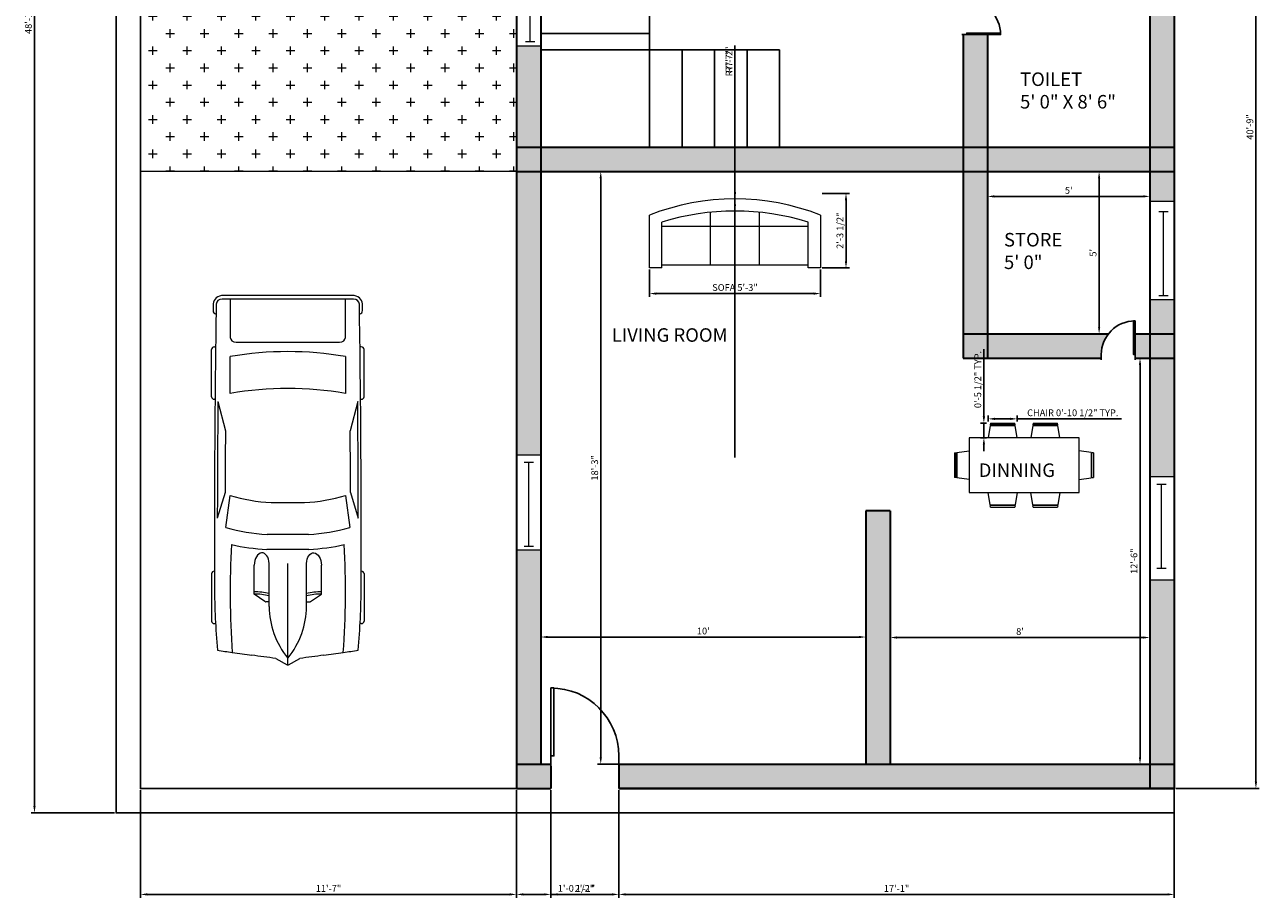
# Model space of a CAD drawing. Units: millimetres. Extents: x 2602 to 3574, y 848 to 1501.
# Tile 1 of 3: x 2602 to 3058, y 848 to 1172. Entities that reach past the tile are written whole.
import ezdxf

# ---------------------------------------------------------------- set-up
doc = ezdxf.new("R2010")
doc.units = ezdxf.units.MM
for name, color, linetype, lineweight in [('A-ANNO-DIMS', 170, 'Continuous', 18), ('A-AREA-IDEN', 200, 'Continuous', 18), ('A-WALL-PATT', 140, 'Continuous', 13), ('C-PROP', 140, 'Continuous', 25), ('C-SITE-VEHI', 90, 'Continuous', 13), ('doors', 10, 'Continuous', 25), ('furniture', 90, 'Continuous', 18), ('L-PLNT', 140, 'Continuous', 18), ('L-PLNT-PATT', 152, 'Continuous', 13), ('STAIRCASE', 30, 'Continuous', 25), ('walls', 140, 'Continuous', 35), ('windows', 40, 'Continuous', 18)]:
    doc.layers.add(name, color=color, linetype=linetype, lineweight=lineweight)
doc.styles.get("Standard").update_dxf_attribs({"font": 'arial.ttf'})
doc.dimstyles.new('ISO-25', dxfattribs={"dimtxt": 2.5, "dimasz": 2.5, "dimexe": 1.25, "dimexo": 0.625, "dimtad": 1, "dimdec": 0, "dimlunit": 3, "dimtxsty": 'Standard', "dimcen": 2.5, "dimadec": 0, "dimazin": 0, "dimtfac": 1, "dimtdec": 0, "dimtmove": 0, "dimatfit": 3, "dimfxl": 1, "dimarcsym": 0})

# ---------------------------------------------------------------- blocks, each defined once
blk = doc.blocks.new('*U2')
for p, q in [((0, 0), (0, -6)), ((40, 0), (40, -6))]:
    blk.add_line(p, q)
blk.add_lwpolyline([(0, 0), (0, 40), (1.75, 40), (1.75, 0)], close=True)
blk.add_arc((0, 0), 40, 0, 90)
blk = doc.blocks.new('*U4')
for p, q in [((0, 4), (0, 0)), ((0, 2), (36, 2)), ((36, 4), (36, 0))]:
    blk.add_line(p, q)
blk = doc.blocks.new('Sofa - Roundback 7 ft.')
for p, q in [((-36.000027, -34), (-36.000027, -11.4696)), ((-12.00002, -32.4421), (-12.00003, -6.5971)), ((11.99997, -32.4421), (11.99998, -6.5971)), ((35.99998, -34), (35.99998, -11.4696)), ((-35.999844, -13.3819), (35.9998, -13.3819)), ((-36.000027, -32.4421), (35.99998, -32.4421))]:
    blk.add_line(p, q)
for points in [[(-36.000027, -34), (-42.000027, -34), (-42.000027, -8)], [(41.99998, -8), (41.99998, -34), (35.99998, -34)]]:
    blk.add_lwpolyline(points)
for centre, radius, start, end in [((0, -114.25), 114.25, 68.43141, 111.5686), ((-0.00001, -127.1968), 121.1968, 72.72033, 107.2797)]:
    blk.add_arc(centre, radius, start, end)
blk = doc.blocks.new('*D13')
at = {"layer": 'A-ANNO-DIMS', "color": 0, "lineweight": -2, "transparency": 16777216}
for p, q in [((2993.44, 1117.36), (3000.35, 1117.36)), ((2999.1, 1114.86), (2999.1, 1059.86)), ((2993.44, 1057.36), (3000.35, 1057.36))]:
    blk.add_line(p, q, dxfattribs=at)
at = {"layer": 'A-ANNO-DIMS', "color": 0, "transparency": 16777216}
for points in [[(2998.69, 1114.86), (2999.52, 1114.86), (2999.1, 1117.36)], [(2998.69, 1059.86), (2999.52, 1059.86), (2999.1, 1057.36)]]:
    blk.add_solid(points, dxfattribs=at)
at = {"layer": 'Defpoints', "color": 0, "transparency": 16777216}
for p in [(2992.82, 1117.36), (2992.82, 1057.36), (2999.1, 1057.36)]:
    blk.add_point(p, dxfattribs=at)
at = {"layer": 'A-ANNO-DIMS', "color": 0, "transparency": 16777216, "insert": (2997.21, 1087.36), "char_height": 2.5, "attachment_point": 5, "rotation": 90}
blk.add_mtext("5'", dxfattribs=at)
blk = doc.blocks.new('*D14')
at = {"layer": 'A-ANNO-DIMS', "color": 0, "lineweight": -2, "transparency": 16777216}
for p, q in [((2957.88, 1110.38), (2957.88, 1106.94)), ((3017.88, 1110.38), (3017.88, 1106.94)), ((3015.38, 1108.19), (2960.38, 1108.19))]:
    blk.add_line(p, q, dxfattribs=at)
at = {"layer": 'A-ANNO-DIMS', "color": 0, "transparency": 16777216}
for points in [[(2960.38, 1108.61), (2960.38, 1107.77), (2957.88, 1108.19)], [(3015.38, 1108.61), (3015.38, 1107.77), (3017.88, 1108.19)]]:
    blk.add_solid(points, dxfattribs=at)
at = {"layer": 'Defpoints', "color": 0, "transparency": 16777216}
for p in [(2957.88, 1111.01), (3017.88, 1111.01), (2957.88, 1108.19)]:
    blk.add_point(p, dxfattribs=at)
at = {"layer": 'A-ANNO-DIMS', "color": 0, "transparency": 16777216, "insert": (2987.88, 1110.09), "char_height": 2.5, "attachment_point": 5}
blk.add_mtext("5'", dxfattribs=at)
blk = doc.blocks.new('*D15')
at = {"layer": 'A-ANNO-DIMS', "color": 0, "lineweight": -2, "transparency": 16777216}
for p, q in [((2921.88, 937.69), (2921.88, 946.41)), ((3015.38, 945.16), (2924.38, 945.16)), ((3017.88, 937.69), (3017.88, 946.41))]:
    blk.add_line(p, q, dxfattribs=at)
at = {"layer": 'A-ANNO-DIMS', "color": 0, "transparency": 16777216}
for points in [[(2924.38, 945.57), (2924.38, 944.74), (2921.88, 945.16)], [(3015.38, 945.57), (3015.38, 944.74), (3017.88, 945.16)]]:
    blk.add_solid(points, dxfattribs=at)
at = {"layer": 'Defpoints', "color": 0, "transparency": 16777216}
for p in [(2921.88, 945.16), (2921.88, 937.07), (3017.88, 937.07)]:
    blk.add_point(p, dxfattribs=at)
at = {"layer": 'A-ANNO-DIMS', "color": 0, "transparency": 16777216, "insert": (2969.88, 947.06), "char_height": 2.5, "attachment_point": 5}
blk.add_mtext("8'", dxfattribs=at)
blk = doc.blocks.new('*D16')
at = {"layer": 'A-ANNO-DIMS', "color": 0, "lineweight": -2, "transparency": 16777216}
for p, q in [((3014.62, 1048.36), (3012.96, 1048.36)), ((3014.21, 1045.86), (3014.21, 900.86)), ((3014.62, 898.36), (3012.96, 898.36))]:
    blk.add_line(p, q, dxfattribs=at)
at = {"layer": 'A-ANNO-DIMS', "color": 0, "transparency": 16777216}
for points in [[(3013.8, 1045.86), (3014.63, 1045.86), (3014.21, 1048.36)], [(3013.8, 900.86), (3014.63, 900.86), (3014.21, 898.36)]]:
    blk.add_solid(points, dxfattribs=at)
at = {"layer": 'Defpoints', "color": 0, "transparency": 16777216}
for p in [(3015.24, 1048.36), (3014.21, 898.36), (3015.24, 898.36)]:
    blk.add_point(p, dxfattribs=at)
at = {"layer": 'A-ANNO-DIMS', "color": 0, "transparency": 16777216, "insert": (3012.31, 973.36), "char_height": 2.5, "attachment_point": 5, "rotation": 90}
blk.add_mtext('12\'-6"', dxfattribs=at)
blk = doc.blocks.new('*D17')
at = {"layer": 'A-ANNO-DIMS', "color": 0, "lineweight": -2, "transparency": 16777216}
for p, q in [((2792.88, 975.8), (2792.88, 944.09)), ((2912.88, 975.8), (2912.88, 944.09)), ((2910.38, 945.34), (2795.38, 945.34))]:
    blk.add_line(p, q, dxfattribs=at)
at = {"layer": 'A-ANNO-DIMS', "color": 0, "transparency": 16777216}
for points in [[(2795.38, 945.76), (2795.38, 944.92), (2792.88, 945.34)], [(2910.38, 945.76), (2910.38, 944.92), (2912.88, 945.34)]]:
    blk.add_solid(points, dxfattribs=at)
at = {"layer": 'Defpoints', "color": 0, "transparency": 16777216}
for p in [(2792.88, 976.43), (2912.88, 976.43), (2792.88, 945.34)]:
    blk.add_point(p, dxfattribs=at)
at = {"layer": 'A-ANNO-DIMS', "color": 0, "transparency": 16777216, "insert": (2852.88, 947.24), "char_height": 2.5, "attachment_point": 5}
blk.add_mtext("10'", dxfattribs=at)
blk = doc.blocks.new('*D18')
at = {"layer": 'A-ANNO-DIMS', "color": 0, "lineweight": -2, "transparency": 16777216}
for p, q in [((2830.28, 1117.36), (2813.75, 1117.36)), ((2815, 900.86), (2815, 1114.86)), ((2830.28, 898.36), (2813.75, 898.36))]:
    blk.add_line(p, q, dxfattribs=at)
at = {"layer": 'A-ANNO-DIMS', "color": 0, "transparency": 16777216}
for points in [[(2814.58, 1114.86), (2815.41, 1114.86), (2815, 1117.36)], [(2814.58, 900.86), (2815.41, 900.86), (2815, 898.36)]]:
    blk.add_solid(points, dxfattribs=at)
at = {"layer": 'Defpoints', "color": 0, "transparency": 16777216}
for p in [(2815, 1117.36), (2830.91, 1117.36), (2830.91, 898.36)]:
    blk.add_point(p, dxfattribs=at)
at = {"layer": 'A-ANNO-DIMS', "color": 0, "transparency": 16777216, "insert": (2813.09, 1007.86), "char_height": 2.5, "attachment_point": 5, "rotation": 90}
blk.add_mtext('18\'-3"', dxfattribs=at)
blk = doc.blocks.new('*U22')
for p, q in [((46.55, 38.89), (22.35, 38.89)), ((136.7, 38.89), (160.9, 38.89)), ((21.1, 37.41), (21.1, 36.83)), ((47.8, 37.39), (47.8, 37.41)), ((70.03, 31.54), (86.41, 29.35)), ((87.99, 31.87), (74.76, 35.92)), ((134.31, 35.6), (119.29, 31.78)), ((135.45, 37.07), (135.45, 37.41)), ((162.15, 37.41), (162.15, 36.77)), ((186.47, -33.5), (186.47, 33.5)), ((188.4, -32.76), (188.4, 32.76)), ((138.42, 29.35), (157.25, 29.35)), ((164.52, 26.39), (164.52, -26.39)), ((186.47, 29.35), (167.01, 29.35)), ((32.27, 11.63), (36.13, 17.17)), ((36.13, 17.17), (50.94, 17.17)), ((29.77, 9.51), (51.68, 9.51)), ((32.12, 9.51), (32.12, 11.15)), ((58.92, -10.77), (58.92, 10.77)), ((66.55, -10.53), (66.55, 10.53)), ((82.74, 8.5), (82.74, -8.5)), ((186.47, -10.53), (186.47, 10.53)), ((3.27, 6.13), (0.1, 0.41)), ((0, 0), (51.68, 0)), ((0.1, -0.41), (3.27, -6.13)), ((29.77, -9.51), (51.68, -9.51)), ((32.12, -9.51), (32.12, -11.15)), ((32.27, -11.63), (36.13, -17.17)), ((36.13, -17.17), (50.94, -17.17)), ((86.41, -29.35), (70.03, -31.54)), ((157.25, -29.35), (138.42, -29.35)), ((167.01, -29.35), (186.47, -29.35)), ((21.1, -37.41), (21.1, -36.83)), ((47.8, -37.39), (47.8, -37.41)), ((87.99, -31.87), (74.76, -35.92)), ((134.31, -35.6), (119.29, -31.78)), ((135.45, -37.07), (135.45, -37.41)), ((162.15, -37.41), (162.15, -36.77)), ((46.55, -38.89), (22.35, -38.89)), ((136.7, -38.89), (160.9, -38.89))]:
    blk.add_line(p, q)
for centre, major_axis, ratio, start_param, end_param in [((22.35, 37.41), (0, -1.48), 0.842304, 3.141593, 4.712389), ((46.55, 37.41), (0, 1.48), 0.842304, -1.570796, 0), ((136.7, 37.41), (0, -1.48), 0.842304, 3.141593, 4.712389), ((160.9, 37.41), (0, 1.48), 0.842304, -1.570796, 0), ((180.63, 35.84), (0, 2.22), 0.842304, -0.013017, 1.249894), ((64.48, -10556.36), (0, 10595.31), 0.842304, -0.013397, -0.013017), ((183.98, 32.76), (0, -5.25), 0.842304, 1.570796, 3.128196), ((266.03, -27.52), (0, 313.31), 0.842304, 1.367076, 1.39176), ((41.19, -490.86), (0, 528.23), 0.842304, 0.00281, 0.075598), ((64.48, -10555.62), (0, 10593.03), 0.842304, -0.013397, 0.002797), ((135.29, 5.39), (0, 81.77), 0.842304, 1.245306, 1.50788), ((64.48, -10555.62), (0, -10591.55), 0.842304, 3.133765, 3.140441), ((95.79, -3666.35), (0, -3698.24), 0.842304, 3.134049, 3.144098), ((183.98, 33.5), (0, -2.96), 0.842304, 1.570796, 3.128196), ((259.18, -27.52), (0, -305.3), 0.842304, 4.528606, 4.561838), ((37.47, -593.96), (0, -623.33), 0.842304, 3.096046, 3.200911), ((134.4, 5.39), (0, -89.78), 0.842304, 4.449482, 4.652344), ((149.6, 2.8), (0, -79.58), 0.842304, 4.372215, 4.640744), ((17.08, 0), (0, 147.02), 0.842304, 4.511394, 4.913384), ((35.91, 0), (0, 147.02), 0.842304, 4.511394, 4.913384), ((167.01, 26.39), (0, 2.96), 0.842304, 0, 1.570796), ((-204.49, 52.4), (0, -250.96), 0.842304, 1.385369, 1.434372), ((13.04, 17.01), (0, 27.42), 0.842304, 4.435146, 4.718221), ((14.2, 17.01), (0, 27.42), 0.842304, 4.435146, 4.718221), ((50.79, 13.34), (6.34, -0.36), 0.603834, -1.395552, 1.581315), ((29.77, -46.66), (0, 56.17), 0.842304, 0, 0.590319), ((32.75, 11.15), (0, 0.74), 0.842304, 0.879714, 1.570796), ((0.62, 0), (0, -0.74), 0.842304, 4.131459, 5.293319), ((-204.49, -52.4), (0, 250.96), 0.842304, -1.434372, -1.385369), ((29.77, 46.66), (0, 56.17), 0.842304, 2.551274, 3.141593), ((32.75, -11.15), (0, -0.74), 0.842304, 4.712389, 5.403472), ((13.04, -17.01), (0, -27.42), 0.842304, 1.564964, 1.848039), ((14.2, -17.01), (0, -27.42), 0.842304, 1.564964, 1.848039), ((134.4, -5.39), (0, -89.78), 0.842304, -1.510751, -1.307889), ((135.29, -5.39), (0, -81.77), 0.842304, -1.50788, -1.245306), ((149.6, -2.8), (0, -79.58), 0.842304, -1.499151, -1.230623), ((259.18, 27.52), (0, 305.3), 0.842304, 1.721348, 1.754579), ((266.03, 27.52), (0, 313.31), 0.842304, 1.749832, 1.774517), ((37.47, 593.96), (0, -623.33), 0.842304, -0.059319, 0.045547), ((167.01, -26.39), (0, -2.96), 0.842304, 4.712389, 6.283185), ((41.19, 490.86), (0, -528.23), 0.842304, -0.075598, -0.00281), ((22.35, -37.41), (0, 1.48), 0.842304, 1.570796, 3.141593), ((64.48, 10555.62), (0, 10593.03), 0.842304, 3.138796, 3.15499), ((46.55, -37.41), (0, -1.48), 0.842304, 0, 1.570796), ((64.48, 10555.62), (0, -10591.55), 0.842304, 0.001152, 0.007828), ((95.79, 3666.35), (0, -3698.24), 0.842304, -0.002505, 0.007544), ((136.7, -37.41), (0, -1.48), 0.842304, -1.570796, 0), ((160.9, -37.41), (0, 1.48), 0.842304, 3.141593, 4.712389), ((180.63, -35.84), (0, -2.22), 0.842304, -1.249894, 0.013017), ((183.98, -33.5), (0, 2.96), 0.842304, 3.15499, 4.712389), ((183.98, -32.76), (0, -5.25), 0.842304, 0.013397, 1.570796), ((64.48, 10556.36), (0, 10595.31), 0.842304, 3.15461, 3.15499)]:
    blk.add_ellipse(centre, major_axis=major_axis, ratio=ratio, start_param=start_param, end_param=end_param)
at = {"extrusion": (0, 0, -1)}
blk.add_ellipse((50.79, -13.34), major_axis=(6.34, 0.36), ratio=0.603834, start_param=-1.395552, end_param=1.581315, dxfattribs=at)
blk = doc.blocks.new('CHAIR-DINING')
for p, q in [((0.84, 5.36), (0.75, 4.79)), ((9.95, 4.79), (0.75, 4.79)), ((0.84, 5.36), (9.86, 5.36)), ((9.95, 4.79), (9.86, 5.36)), ((0.71, 4.51), (0, 0)), ((0.71, 4.51), (9.99, 4.51)), ((10.7, 0), (9.99, 4.51))]:
    blk.add_line(p, q)
blk = doc.blocks.new('*D26')
at = {"layer": 'A-ANNO-DIMS', "color": 0, "lineweight": -2, "transparency": 16777216}
for p, q in [((2958.13, 1024.99), (2958.13, 1027.22)), ((2968.83, 1024.99), (2968.83, 1027.22)), ((2960.63, 1025.97), (2966.33, 1025.97)), ((2968.83, 1025.97), (3007.39, 1025.97))]:
    blk.add_line(p, q, dxfattribs=at)
at = {"layer": 'A-ANNO-DIMS', "color": 0, "transparency": 16777216}
for points in [[(2960.63, 1026.39), (2960.63, 1025.56), (2958.13, 1025.97)], [(2966.33, 1026.39), (2966.33, 1025.56), (2968.83, 1025.97)]]:
    blk.add_solid(points, dxfattribs=at)
at = {"layer": 'Defpoints', "color": 0, "transparency": 16777216}
for p in [(2958.13, 1024.37), (2968.83, 1025.97), (2968.83, 1024.37)]:
    blk.add_point(p, dxfattribs=at)
at = {"layer": 'A-ANNO-DIMS', "color": 0, "transparency": 16777216, "insert": (2989.36, 1027.89), "char_height": 2.5, "attachment_point": 5}
blk.add_mtext('CHAIR 0\'-10 1/2" TYP.', dxfattribs=at)
blk = doc.blocks.new('*D27')
at = {"layer": 'A-ANNO-DIMS', "color": 0, "lineweight": -2, "transparency": 16777216}
for p, q in [((2956.53, 1026.87), (2956.53, 1051.68)), ((2957.51, 1024.37), (2955.28, 1024.37)), ((2956.53, 1019.01), (2956.53, 1024.37)), ((2957.51, 1019.01), (2955.28, 1019.01)), ((2956.53, 1016.51), (2956.53, 1014.01))]:
    blk.add_line(p, q, dxfattribs=at)
at = {"layer": 'A-ANNO-DIMS', "color": 0, "transparency": 16777216}
for points in [[(2956.11, 1026.87), (2956.95, 1026.87), (2956.53, 1024.37)], [(2956.11, 1016.51), (2956.95, 1016.51), (2956.53, 1019.01)]]:
    blk.add_solid(points, dxfattribs=at)
at = {"layer": 'Defpoints', "color": 0, "transparency": 16777216}
for p in [(2956.53, 1024.37), (2958.13, 1024.37), (2958.13, 1019.01)]:
    blk.add_point(p, dxfattribs=at)
at = {"layer": 'A-ANNO-DIMS', "color": 0, "transparency": 16777216, "insert": (2954.61, 1040.52), "char_height": 2.5, "attachment_point": 5, "rotation": 90}
blk.add_mtext('0\'-5 1/2" TYP.', dxfattribs=at)
blk = doc.blocks.new('*D36')
at = {"layer": 'A-ANNO-DIMS', "color": 0, "lineweight": -2, "transparency": 16777216}
for p, q in [((2833.05, 1081.12), (2833.05, 1071.03)), ((2896.14, 1081.12), (2896.14, 1071.03)), ((2835.55, 1072.28), (2893.64, 1072.28))]:
    blk.add_line(p, q, dxfattribs=at)
at = {"layer": 'A-ANNO-DIMS', "color": 0, "transparency": 16777216}
for points in [[(2835.55, 1072.7), (2835.55, 1071.86), (2833.05, 1072.28)], [(2893.64, 1072.7), (2893.64, 1071.86), (2896.14, 1072.28)]]:
    blk.add_solid(points, dxfattribs=at)
at = {"layer": 'Defpoints', "color": 0, "transparency": 16777216}
for p in [(2833.05, 1081.74), (2896.14, 1081.74), (2896.14, 1072.28)]:
    blk.add_point(p, dxfattribs=at)
at = {"layer": 'A-ANNO-DIMS', "color": 0, "transparency": 16777216, "insert": (2864.59, 1074.2), "char_height": 2.5, "attachment_point": 5}
blk.add_mtext('SOFA 5\'-3"', dxfattribs=at)
blk = doc.blocks.new('*D37')
at = {"layer": 'A-ANNO-DIMS', "color": 0, "lineweight": -2, "transparency": 16777216}
for p, q in [((2896.76, 1109.28), (2906.85, 1109.28)), ((2905.6, 1084.24), (2905.6, 1106.78)), ((2896.76, 1081.74), (2906.85, 1081.74))]:
    blk.add_line(p, q, dxfattribs=at)
at = {"layer": 'A-ANNO-DIMS', "color": 0, "transparency": 16777216}
for points in [[(2905.18, 1106.78), (2906.01, 1106.78), (2905.6, 1109.28)], [(2905.18, 1084.24), (2906.01, 1084.24), (2905.6, 1081.74)]]:
    blk.add_solid(points, dxfattribs=at)
at = {"layer": 'Defpoints', "color": 0, "transparency": 16777216}
for p in [(2896.14, 1109.28), (2905.6, 1109.28), (2896.14, 1081.74)]:
    blk.add_point(p, dxfattribs=at)
at = {"layer": 'A-ANNO-DIMS', "color": 0, "transparency": 16777216, "insert": (2903.68, 1095.51), "char_height": 2.5, "attachment_point": 5, "rotation": 90}
blk.add_mtext('2\'-3 1/2"', dxfattribs=at)
blk = doc.blocks.new('*D41')
at = {"layer": 'A-ANNO-DIMS', "color": 0, "lineweight": -2, "transparency": 16777216}
for p, q in [((2635.33, 1467.39), (2604.55, 1467.39)), ((2605.8, 882.86), (2605.8, 1464.89)), ((2635.33, 880.36), (2604.55, 880.36))]:
    blk.add_line(p, q, dxfattribs=at)
at = {"layer": 'A-ANNO-DIMS', "color": 0, "transparency": 16777216}
for points in [[(2605.39, 1464.89), (2606.22, 1464.89), (2605.8, 1467.39)], [(2605.39, 882.86), (2606.22, 882.86), (2605.8, 880.36)]]:
    blk.add_solid(points, dxfattribs=at)
at = {"layer": 'Defpoints', "color": 0, "transparency": 16777216}
for p in [(2605.8, 1467.39), (2635.95, 1467.39), (2635.95, 880.36)]:
    blk.add_point(p, dxfattribs=at)
at = {"layer": 'A-ANNO-DIMS', "color": 0, "transparency": 16777216, "insert": (2603.9, 1173.88), "char_height": 2.5, "attachment_point": 5, "rotation": 90}
blk.add_mtext('48\'-11"', dxfattribs=at)
blk = doc.blocks.new('*D42')
at = {"layer": 'A-ANNO-DIMS', "color": 0, "lineweight": -2, "transparency": 16777216}
for p, q in [((3027.5, 1378.36), (3058.28, 1378.36)), ((3057.03, 891.86), (3057.03, 1375.86)), ((3027.5, 889.36), (3058.28, 889.36))]:
    blk.add_line(p, q, dxfattribs=at)
at = {"layer": 'A-ANNO-DIMS', "color": 0, "transparency": 16777216}
for points in [[(3056.61, 1375.86), (3057.44, 1375.86), (3057.03, 1378.36)], [(3056.61, 891.86), (3057.44, 891.86), (3057.03, 889.36)]]:
    blk.add_solid(points, dxfattribs=at)
at = {"layer": 'Defpoints', "color": 0, "transparency": 16777216}
for p in [(3026.88, 1378.36), (3057.03, 1378.36), (3026.88, 889.36)]:
    blk.add_point(p, dxfattribs=at)
at = {"layer": 'A-ANNO-DIMS', "color": 0, "transparency": 16777216, "insert": (3055.12, 1133.86), "char_height": 2.5, "attachment_point": 5, "rotation": 90}
blk.add_mtext('40\'-9"', dxfattribs=at)
blk = doc.blocks.new('*D44')
at = {"layer": 'A-ANNO-DIMS', "color": 0, "lineweight": -2, "transparency": 16777216}
for p, q in [((2644.95, 888.74), (2644.95, 848.96)), ((2783.88, 888.74), (2783.88, 848.96)), ((2647.45, 850.21), (2781.38, 850.21))]:
    blk.add_line(p, q, dxfattribs=at)
at = {"layer": 'A-ANNO-DIMS', "color": 0, "transparency": 16777216}
for points in [[(2647.45, 850.63), (2647.45, 849.8), (2644.95, 850.21)], [(2781.38, 850.63), (2781.38, 849.8), (2783.88, 850.21)]]:
    blk.add_solid(points, dxfattribs=at)
at = {"layer": 'Defpoints', "color": 0, "transparency": 16777216}
for p in [(2644.95, 889.36), (2783.88, 889.36), (2783.88, 850.21)]:
    blk.add_point(p, dxfattribs=at)
at = {"layer": 'A-ANNO-DIMS', "color": 0, "transparency": 16777216, "insert": (2714.42, 852.09), "char_height": 2.5, "attachment_point": 5}
blk.add_mtext('11\'-7"', dxfattribs=at)
blk = doc.blocks.new('*D45')
at = {"layer": 'A-ANNO-DIMS', "color": 0, "lineweight": -2, "transparency": 16777216}
for p, q in [((2783.88, 888.74), (2783.88, 848.96)), ((2796.6, 888.74), (2796.6, 848.96)), ((2786.38, 850.21), (2794.1, 850.21)), ((2796.6, 850.21), (2812.58, 850.21))]:
    blk.add_line(p, q, dxfattribs=at)
at = {"layer": 'A-ANNO-DIMS', "color": 0, "transparency": 16777216}
for points in [[(2786.38, 850.63), (2786.38, 849.8), (2783.88, 850.21)], [(2794.1, 850.63), (2794.1, 849.8), (2796.6, 850.21)]]:
    blk.add_solid(points, dxfattribs=at)
at = {"layer": 'Defpoints', "color": 0, "transparency": 16777216}
for p in [(2783.88, 889.36), (2796.6, 889.36), (2796.6, 850.21)]:
    blk.add_point(p, dxfattribs=at)
at = {"layer": 'A-ANNO-DIMS', "color": 0, "transparency": 16777216, "insert": (2805.84, 852.13), "char_height": 2.5, "attachment_point": 5}
blk.add_mtext('1\'-0 1/2"', dxfattribs=at)
blk = doc.blocks.new('*D46')
at = {"layer": 'A-ANNO-DIMS', "color": 0, "lineweight": -2, "transparency": 16777216}
for p, q in [((2796.6, 888.74), (2796.6, 848.96)), ((2821.68, 888.74), (2821.68, 848.96)), ((2799.1, 850.21), (2819.18, 850.21))]:
    blk.add_line(p, q, dxfattribs=at)
at = {"layer": 'A-ANNO-DIMS', "color": 0, "transparency": 16777216}
for points in [[(2799.1, 850.63), (2799.1, 849.8), (2796.6, 850.21)], [(2819.18, 850.63), (2819.18, 849.8), (2821.68, 850.21)]]:
    blk.add_solid(points, dxfattribs=at)
at = {"layer": 'Defpoints', "color": 0, "transparency": 16777216}
for p in [(2796.6, 889.36), (2821.68, 889.36), (2821.68, 850.21)]:
    blk.add_point(p, dxfattribs=at)
at = {"layer": 'A-ANNO-DIMS', "color": 0, "transparency": 16777216, "insert": (2809.14, 852.09), "char_height": 2.5, "attachment_point": 5}
blk.add_mtext('2\'-1"', dxfattribs=at)
blk = doc.blocks.new('*D47')
at = {"layer": 'A-ANNO-DIMS', "color": 0, "lineweight": -2, "transparency": 16777216}
for p, q in [((2821.68, 888.74), (2821.68, 848.96)), ((3026.88, 888.74), (3026.88, 848.96)), ((2824.18, 850.21), (3024.38, 850.21))]:
    blk.add_line(p, q, dxfattribs=at)
at = {"layer": 'A-ANNO-DIMS', "color": 0, "transparency": 16777216}
for points in [[(2824.18, 850.63), (2824.18, 849.8), (2821.68, 850.21)], [(3024.38, 850.63), (3024.38, 849.8), (3026.88, 850.21)]]:
    blk.add_solid(points, dxfattribs=at)
at = {"layer": 'Defpoints', "color": 0, "transparency": 16777216}
for p in [(2821.68, 889.36), (3026.88, 889.36), (3026.88, 850.21)]:
    blk.add_point(p, dxfattribs=at)
at = {"layer": 'A-ANNO-DIMS', "color": 0, "transparency": 16777216, "insert": (2924.28, 852.09), "char_height": 2.5, "attachment_point": 5}
blk.add_mtext('17\'-1"', dxfattribs=at)
blk = doc.blocks.new('*D57')
at = {"layer": 'A-ANNO-DIMS', "color": 0, "lineweight": -2, "transparency": 16777216}
for p, q in [((2864.59, 1162.53), (2864.59, 1105.27)), ((2864.59, 1011.75), (2864.59, 1102.77))]:
    blk.add_line(p, q, dxfattribs=at)
at = {"layer": 'A-ANNO-DIMS', "color": 0, "transparency": 16777216}
blk.add_solid([(2864.18, 1105.27), (2865.01, 1105.27), (2864.59, 1102.77)], dxfattribs=at)
at = {"layer": 'Defpoints', "color": 0, "transparency": 16777216}
for p in [(2864.59, 1102.77), (2864.59, 1011.75)]:
    blk.add_point(p, dxfattribs=at)
at = {"layer": 'A-ANNO-DIMS', "color": 0, "transparency": 16777216, "insert": (2862.72, 1157.39), "char_height": 2.5, "attachment_point": 5, "rotation": 89.9998}
blk.add_mtext('R7\'-7"', dxfattribs=at)
blk = doc.blocks.new('*D58')
at = {"layer": 'A-ANNO-DIMS', "color": 0, "lineweight": -2, "transparency": 16777216}
for p, q in [((2864.59, 1163.91), (2864.59, 1109.78)), ((2864.59, 1021.47), (2864.59, 1107.28))]:
    blk.add_line(p, q, dxfattribs=at)
at = {"layer": 'A-ANNO-DIMS', "color": 0, "transparency": 16777216}
blk.add_solid([(2864.18, 1109.78), (2865.01, 1109.78), (2864.59, 1107.28)], dxfattribs=at)
at = {"layer": 'Defpoints', "color": 0, "transparency": 16777216}
for p in [(2864.59, 1107.28), (2864.59, 1021.47)]:
    blk.add_point(p, dxfattribs=at)
at = {"layer": 'A-ANNO-DIMS', "color": 0, "transparency": 16777216, "insert": (2862.71, 1158.76), "char_height": 2.5, "attachment_point": 5, "rotation": 89.9998}
blk.add_mtext('R7\'-2"', dxfattribs=at)

msp = doc.modelspace()

# ---------------------------------------------------------------- hatches: boundary and pattern name
at = {"layer": 'A-WALL-PATT'}
h = msp.add_hatch(color=256, dxfattribs=at)
h.dxf.hatch_style = 1
h.paths.add_polyline_path([(2792.88, 1117.36), (2783.88, 1117.36), (2783.88, 1012.52), (2792.88, 1012.52)])
h.paths.add_polyline_path([(2957.88, 1117.36), (2948.88, 1117.36), (2948.88, 1057.36), (2957.88, 1057.36)])
h.paths.add_polyline_path([(2957.88, 1057.36), (2948.88, 1057.36), (2948.88, 1048.36), (2957.88, 1048.36)])
h.paths.add_polyline_path([(3002.51, 1057.36), (2957.88, 1057.36), (2957.88, 1048.36), (2999.91, 1048.36), (2999.91, 1049.72, -0.166059)])
h.paths.add_polyline_path([(3026.88, 1057.36), (3017.88, 1057.36), (3017.88, 1048.36), (3026.88, 1048.36)])
h.paths.add_polyline_path([(3017.88, 1057.36), (3012.39, 1057.36), (3012.39, 1049.72), (3012.39, 1048.36), (3017.88, 1048.36)])
h.paths.add_polyline_path([(3026.88, 1048.36), (3017.88, 1048.36), (3017.88, 1004.59), (3026.88, 1004.59)])
h.paths.add_polyline_path([(3026.88, 1069.96), (3017.88, 1069.96), (3017.88, 1057.36), (3026.88, 1057.36)])
h.paths.add_polyline_path([(3017.88, 1126.36), (2957.88, 1126.36), (2957.88, 1117.36), (3017.88, 1117.36)])
h.paths.add_polyline_path([(2957.88, 1126.36), (2948.88, 1126.36), (2948.88, 1117.36), (2957.88, 1117.36)])
h.paths.add_polyline_path([(2948.88, 1126.36), (2792.88, 1126.36), (2792.88, 1117.36), (2948.88, 1117.36)])
h.paths.add_polyline_path([(2957.88, 1168.02), (2950.23, 1168.02), (2948.88, 1168.02), (2948.88, 1126.36), (2957.88, 1126.36)])
h.paths.add_polyline_path([(3026.88, 1176.14), (3017.88, 1176.14), (3017.88, 1126.36), (3026.88, 1126.36)])
h.paths.add_polyline_path([(3026.88, 1126.36), (3017.88, 1126.36), (3017.88, 1117.36), (3026.88, 1117.36)])
h.paths.add_polyline_path([(3026.88, 1117.36), (3017.88, 1117.36), (3017.88, 1106.26), (3026.88, 1106.26)])
h.paths.add_polyline_path([(2792.88, 1163.71), (2783.88, 1163.71), (2783.88, 1126.36), (2792.88, 1126.36)])
h.paths.add_polyline_path([(2792.88, 1126.36), (2783.88, 1126.36), (2783.88, 1117.36), (2792.88, 1117.36)])
h.paths.add_polyline_path([(2921.88, 991.95), (2912.88, 991.95), (2912.88, 898.36), (2921.88, 898.36)])
h.paths.add_polyline_path([(3026.88, 966.36), (3017.88, 966.36), (3017.88, 898.36), (3026.88, 898.36)])
h.paths.add_polyline_path([(2792.88, 977.5), (2783.88, 977.5), (2783.88, 898.36), (2792.88, 898.36)])
h.paths.add_polyline_path([(2792.88, 1228.36), (2783.88, 1228.36), (2783.88, 1198.24), (2792.88, 1198.24)])
h.paths.add_polyline_path([(2792.88, 1290.09), (2783.88, 1290.09), (2783.88, 1237.36), (2792.88, 1237.36)])
h.paths.add_polyline_path([(2792.88, 1237.36), (2783.88, 1237.36), (2783.88, 1228.36), (2792.88, 1228.36)])
h.paths.add_polyline_path([(2948.88, 1378.36), (2792.88, 1378.36), (2792.88, 1369.36), (2948.88, 1369.36)])
h.paths.add_polyline_path([(2792.88, 1378.36), (2783.88, 1378.36), (2783.88, 1369.36), (2792.88, 1369.36)])
h.paths.add_polyline_path([(2792.88, 1369.36), (2783.88, 1369.36), (2783.88, 1326.82), (2792.88, 1326.82)])
h.paths.add_polyline_path([(2957.88, 1347.96, -0.166257), (2950.23, 1345.35), (2948.88, 1345.35), (2948.88, 1237.36), (2957.88, 1237.36)])
h.paths.add_polyline_path([(3017.88, 1237.36), (2957.88, 1237.36), (2957.88, 1228.36), (3017.88, 1228.36)])
h.paths.add_polyline_path([(2957.88, 1237.36), (2948.88, 1237.36), (2948.88, 1228.36), (2957.88, 1228.36)])
h.paths.add_polyline_path([(2948.88, 1237.36), (2943.82, 1237.36, -0.076419), (2944.98, 1229.83), (2944.98, 1228.36), (2948.88, 1228.36)])
h.paths.add_polyline_path([(3026.88, 1237.36), (3017.88, 1237.36), (3017.88, 1228.36), (3026.88, 1228.36)])
h.paths.add_polyline_path([(3026.88, 1285.23), (3017.88, 1285.23), (3017.88, 1237.36), (3026.88, 1237.36)])
h.paths.add_polyline_path([(3026.88, 1228.36), (3017.88, 1228.36), (3017.88, 1214.51), (3026.88, 1214.51)])
h.paths.add_polyline_path([(2919.9, 1237.36), (2792.88, 1237.36), (2792.88, 1228.36), (2919.9, 1228.36), (2919.9, 1229.83)])
h.paths.add_polyline_path([(2957.88, 1228.36), (2948.88, 1228.36), (2948.88, 1180.5), (2950.23, 1180.5, -0.166257), (2957.88, 1177.89)])
h.paths.add_polyline_path([(3026.88, 1369.36), (3017.88, 1369.36), (3017.88, 1319.81), (3026.88, 1319.81)])
h.paths.add_polyline_path([(3026.88, 1378.36), (3017.88, 1378.36), (3017.88, 1369.36), (3026.88, 1369.36)])
h.paths.add_polyline_path([(3017.88, 1378.36), (2957.88, 1378.36), (2957.88, 1369.36), (3017.88, 1369.36)])
h.paths.add_polyline_path([(2957.88, 1378.36), (2948.88, 1378.36), (2948.88, 1369.36), (2957.88, 1369.36)])
h.paths.add_polyline_path([(2957.88, 1369.36), (2948.88, 1369.36), (2948.88, 1357.83), (2950.23, 1357.83), (2957.88, 1357.83)])
h = msp.add_hatch(color=256, dxfattribs=at)
h.dxf.hatch_style = 1
h.paths.add_polyline_path([(2796.6, 897.67), (2796.6, 898.36), (2783.88, 898.36), (2783.88, 889.36), (2796.6, 889.36)])
h.paths.add_polyline_path([(3017.88, 898.36), (2821.68, 898.36), (2821.68, 889.36), (3017.88, 889.36)])
h = msp.add_hatch(color=256, dxfattribs=at)
h.dxf.hatch_style = 1
h.paths.add_polyline_path([(3026.88, 898.36), (3017.88, 898.36), (3017.88, 889.36), (3026.88, 889.36)])
at = {"layer": 'L-PLNT-PATT'}
h = msp.add_hatch(dxfattribs=at)
h.set_pattern_fill('CROSS', color=256)
h.paths.add_polyline_path([(3017.88, 1458.39), (2644.95, 1458.39), (2644.95, 1117.36), (2783.88, 1117.36), (2783.88, 1378.36), (3017.88, 1378.36)])

# ---------------------------------------------------------------- linework, layer by layer
at = {"layer": 'C-PROP'}
msp.add_line((3026.88, 889.36), (3026.88, 880.36), dxfattribs=at)
for points in [[(2796.6, 880.36), (2635.95, 880.36), (2635.95, 1467.39), (3026.88, 1467.39)], [(2796.6, 889.36), (2644.95, 889.36), (2644.95, 1458.39), (3026.88, 1458.39)], [(3026.88, 880.36), (2635.95, 880.36)]]:
    msp.add_lwpolyline(points, dxfattribs=at)
at = {"layer": 'furniture'}
for p, q in [((2991.68, 1019.01), (2951.08, 1019.01)), ((2951.08, 1019.01), (2951.08, 998.71)), ((2991.68, 998.71), (2991.68, 1019.01)), ((2951.08, 998.71), (2991.68, 998.71))]:
    msp.add_line(p, q, dxfattribs=at)
at = {"layer": 'L-PLNT'}
msp.add_line((2783.88, 1117.36), (2644.95, 1117.36), dxfattribs=at)
at = {"layer": 'STAIRCASE'}
for p, q in [((2833.03, 1126.36), (2833.03, 1228.36)), ((2833.03, 1168.36), (2792.88, 1168.36)), ((2881.03, 1162.36), (2792.88, 1162.36)), ((2845.03, 1126.36), (2845.03, 1162.36)), ((2857.03, 1126.36), (2857.03, 1162.36)), ((2869.03, 1126.36), (2869.03, 1162.36)), ((2881.03, 1126.36), (2881.03, 1162.36))]:
    msp.add_line(p, q, dxfattribs=at)
at = {"layer": 'walls'}
for p, q in [((2783.88, 1378.36), (2783.88, 898.36)), ((2792.88, 1378.36), (2792.88, 898.36)), ((3017.88, 1378.36), (3017.88, 889.36)), ((3026.88, 1378.36), (3026.88, 889.36)), ((2948.88, 1168.02), (2948.88, 1048.36)), ((2957.88, 1168.02), (2957.88, 1048.36)), ((2783.88, 1126.36), (3026.88, 1126.36)), ((2783.88, 1117.36), (3026.88, 1117.36)), ((2948.88, 1057.36), (3002.51, 1057.36)), ((3012.39, 1057.36), (3026.88, 1057.36)), ((2948.88, 1048.36), (2999.91, 1048.36)), ((3012.39, 1048.36), (3026.88, 1048.36)), ((2912.88, 991.95), (2912.88, 898.36)), ((2921.88, 991.95), (2912.88, 991.95)), ((2921.88, 991.95), (2921.88, 898.36)), ((2783.88, 898.36), (2796.6, 898.36)), ((2783.88, 898.36), (2783.88, 889.36)), ((2796.6, 897.67), (2796.6, 889.36)), ((2821.68, 898.36), (3026.88, 898.36)), ((2821.68, 898.36), (2821.68, 889.36)), ((2783.88, 889.36), (2796.6, 889.36)), ((2821.68, 889.36), (3026.88, 889.36))]:
    msp.add_line(p, q, dxfattribs=at)
msp.add_lwpolyline([(3026.88, 1378.36), (3026.88, 889.36), (2821.68, 889.36)], dxfattribs=at)
at = {"layer": 'windows'}
for p, q in [((2792.88, 1163.71), (2783.88, 1163.71)), ((3026.88, 1106.26), (3017.88, 1106.26)), ((3026.88, 1069.96), (3017.88, 1069.96)), ((2792.88, 1012.52), (2783.88, 1012.52)), ((3026.88, 1004.59), (3017.88, 1004.59)), ((2792.88, 977.5), (2783.88, 977.5)), ((3026.88, 966.36), (3017.88, 966.36))]:
    msp.add_line(p, q, dxfattribs=at)

# ---------------------------------------------------------------- block references
at = {"layer": 'C-SITE-VEHI', "xscale": 0.7249711451762226, "yscale": 0.7249711451762226, "zscale": 0.7249711451762226, "rotation": 90}
msp.add_blockref('*U22', (2699.4, 935.02), dxfattribs=at)
at = {"layer": 'doors', "xscale": -0.3120057346177813, "yscale": 0.3120057346177813, "zscale": 0.3120057346177813, "rotation": 270}
msp.add_blockref('*U2', (2950.23, 1168.02), dxfattribs=at)
at = {"layer": 'doors'}
for p, xscale, yscale, zscale in [((3012.39, 1049.72), -0.3120057346177813, 0.3120057346177813, 0.3120057346177813), ((2796.6, 901.43), 0.6269655396628341, 0.6269655396628341, 0.6269655396628341)]:
    msp.add_blockref('*U2', p, dxfattribs=dict(at, xscale=xscale, yscale=yscale, zscale=zscale))
at = {"layer": 'furniture', "xscale": 0.751037410380932, "yscale": 0.751037410380932, "zscale": 0.751037410380932}
msp.add_blockref('Sofa - Roundback 7 ft.', (2864.59, 1107.28), dxfattribs=at)
at = {"layer": 'furniture'}
for p in [(2958.13, 1019.01), (2973.92, 1019.01)]:
    msp.add_blockref('CHAIR-DINING', p, dxfattribs=at)
at = {"layer": 'furniture', "extrusion": (0, 0, -1), "zscale": -1}
for p, rotation in [((-2951.08, 1014.21), 270), ((-2958.13, 998.71), 180), ((-2973.92, 998.71), 180)]:
    msp.add_blockref('CHAIR-DINING', p, dxfattribs=dict(at, rotation=rotation))
at = {"layer": 'furniture', "rotation": 270}
msp.add_blockref('CHAIR-DINING', (2991.68, 1014.21), dxfattribs=at)
at = {"layer": 'windows', "xscale": 0.8623741926751115, "yscale": 0.8623741926751115, "zscale": 0.8623741926751115, "rotation": 90}
for p in [(2790.62, 1165.47), (3024.55, 1071.61), (2790.1, 978.93), (3023.82, 970.8)]:
    msp.add_blockref('*U4', p, dxfattribs=at)

# ---------------------------------------------------------------- texts
at = {"layer": 'A-AREA-IDEN', "char_height": 5, "attachment_point": 1}
for s, width, insert in [('TOILET \\P5\' 0" X 8\' 6"', 43.2088, (2969.9, 1154.01)), ('STORE \\P5\' 0"', 45.0278, (2963.96, 1094.68)), ('LIVING ROOM ', 70.3294, (2819.09, 1059.46)), ('DINNING ', 34.3834, (2954.62, 1009.5))]:
    msp.add_mtext_dynamic_manual_height_columns(s, width=width, gutter_width=12.5, heights=[0], dxfattribs=dict(at, insert=insert))

# ---------------------------------------------------------------- dimensions: what is measured, and where the dimension line sits
at = {"layer": 'A-ANNO-DIMS'}
for base, p1, p2, override, picture, middle in [((2605.8, 1467.39), (2635.95, 880.36), (2635.95, 1467.39), {"dimdec": 1, "dimlfac": 1, "dimrnd": 0, "dimzin": 1, "dimdsep": 46, "dimlunit": 4, "dimfrac": 2}, '*D41', (2603.9, 1173.88)), ((3057.03, 1378.36), (3026.88, 889.36), (3026.88, 1378.36), {"dimdec": 1, "dimlfac": 1, "dimrnd": 0, "dimzin": 1, "dimdsep": 46, "dimlunit": 4, "dimfrac": 2}, '*D42', (3055.12, 1133.86)), ((2815, 1117.36), (2830.91, 898.36), (2830.91, 1117.36), {"dimclrd": 0, "dimclre": 0, "dimclrt": 0}, '*D18', (2813.09, 1007.86)), ((2999.1, 1057.36), (2992.82, 1117.36), (2992.82, 1057.36), {"dimclrd": 0, "dimclre": 0, "dimclrt": 0}, '*D13', (2997.21, 1087.36)), ((2905.6, 1109.28), (2896.14, 1081.74), (2896.14, 1109.28), {"dimdec": 1, "dimlfac": 1, "dimrnd": 0, "dimzin": 1, "dimdsep": 46, "dimlunit": 4, "dimfrac": 2}, '*D37', (2903.68, 1095.51)), ((3014.21, 898.36), (3015.24, 1048.36), (3015.24, 898.36), {"dimclrd": 0, "dimclre": 0, "dimclrt": 0}, '*D16', (3012.31, 973.36))]:
    dim = msp.add_linear_dim(base=base, p1=p1, p2=p2, angle=90, dimstyle='ISO-25', override=override, dxfattribs=at)
    dim.commit()
    dim.dimension.update_dxf_attribs({"geometry": picture, "text_midpoint": middle})
for center, mpoint, picture, middle in [((2864.59, 1021.47), (2864.59, 1107.28), '*D58', (2864.59, 1158.76)), ((2864.59, 1011.75), (2864.59, 1102.77), '*D57', (2864.59, 1157.39))]:
    dim = msp.add_radius_dim(center=center, mpoint=mpoint, dimstyle='ISO-25', override={"dimdec": 1, "dimlfac": 1, "dimrnd": 0, "dimzin": 1, "dimdsep": 46, "dimlunit": 4, "dimfrac": 2}, dxfattribs=at)
    dim.commit()
    dim.dimension.update_dxf_attribs({"geometry": picture, "text_midpoint": middle, "dimtype": 164})
for base, p1, p2, override, picture, middle in [((2957.88, 1108.19), (3017.88, 1111.01), (2957.88, 1111.01), {"dimclrd": 0, "dimclre": 0, "dimclrt": 0}, '*D14', (2987.88, 1110.09)), ((2792.88, 945.34), (2912.88, 976.43), (2792.88, 976.43), {"dimclrd": 0, "dimclre": 0, "dimclrt": 0}, '*D17', (2852.88, 947.24)), ((2921.88, 945.16), (3017.88, 937.07), (2921.88, 937.07), {"dimclrd": 0, "dimclre": 0, "dimclrt": 0}, '*D15', (2969.88, 947.06)), ((2783.88, 850.21), (2644.95, 889.36), (2783.88, 889.36), {"dimdec": 1, "dimlfac": 1, "dimrnd": 0, "dimzin": 1, "dimdsep": 46, "dimlunit": 4, "dimfrac": 2}, '*D44', (2714.42, 852.09)), ((2796.6, 850.21), (2783.88, 889.36), (2796.6, 889.36), {"dimdec": 1, "dimlfac": 1, "dimrnd": 0, "dimzin": 1, "dimdsep": 46, "dimlunit": 4, "dimfrac": 2}, '*D45', (2805.84, 852.13)), ((2821.68, 850.21), (2796.6, 889.36), (2821.68, 889.36), {"dimdec": 1, "dimlfac": 1, "dimrnd": 0, "dimzin": 1, "dimdsep": 46, "dimlunit": 4, "dimfrac": 2}, '*D46', (2809.14, 852.09)), ((3026.88, 850.21), (2821.68, 889.36), (3026.88, 889.36), {"dimdec": 1, "dimlfac": 1, "dimrnd": 0, "dimzin": 1, "dimdsep": 46, "dimlunit": 4, "dimfrac": 2}, '*D47', (2924.28, 852.09))]:
    dim = msp.add_linear_dim(base=base, p1=p1, p2=p2, dimstyle='ISO-25', override=override, dxfattribs=at)
    dim.commit()
    dim.dimension.update_dxf_attribs({"geometry": picture, "text_midpoint": middle})
for base, p1, p2, text, picture, middle in [((2896.14, 1072.28), (2833.05, 1081.74), (2896.14, 1081.74), 'SOFA <>', '*D36', (2864.59, 1074.2)), ((2968.83, 1025.97), (2958.13, 1024.37), (2968.83, 1024.37), 'CHAIR <> TYP.', '*D26', (2989.36, 1027.89))]:
    dim = msp.add_linear_dim(base=base, p1=p1, p2=p2, text=text, dimstyle='ISO-25', override={"dimdec": 1, "dimlfac": 1, "dimrnd": 0, "dimzin": 1, "dimdsep": 46, "dimlunit": 4, "dimfrac": 2}, dxfattribs=at)
    dim.commit()
    dim.dimension.update_dxf_attribs({"geometry": picture, "text_midpoint": middle})
dim = msp.add_linear_dim(base=(2956.53, 1024.37), p1=(2958.13, 1019.01), p2=(2958.13, 1024.37), angle=90, text='<> TYP.', dimstyle='ISO-25', override={"dimdec": 1, "dimlfac": 1, "dimrnd": 0, "dimzin": 1, "dimdsep": 46, "dimlunit": 4, "dimfrac": 2}, dxfattribs=at)
dim.commit()
dim.dimension.update_dxf_attribs({"geometry": '*D27', "text_midpoint": (2954.61, 1040.52)})

doc.saveas('drawing.dxf')
